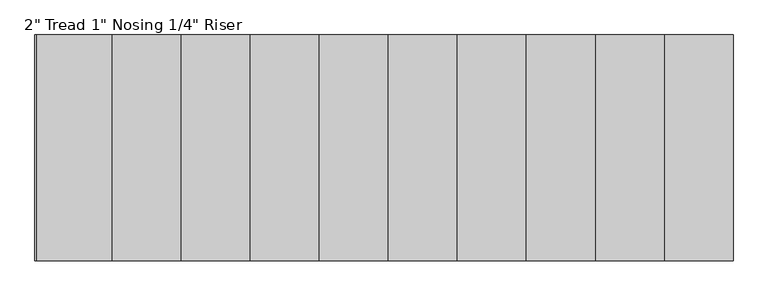
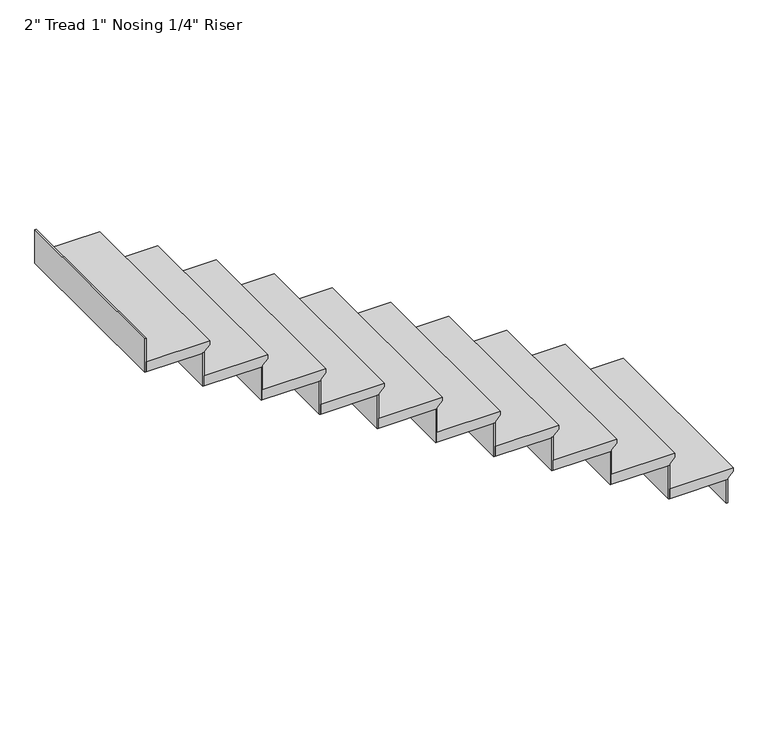
"""IFC4 building model written with IfcOpenShell, lengths in millimetres: stair flight geometry."""

from ifc_helpers import new_model, si_unit, origin, place, context, project, spatial, faceted_brep, source, transform, mapped, element, save


def stair_flight_26c172ca(model_context):
    return source(origin(), model_context, "Body", "Brep", [
        faceted_brep([(-5990.8517085, 2919.0826226, 455.0833333), (-5990.8517085, 2919.0826226, 474.1333333), (-5990.8517085, 2004.6826226, 474.1333333), (-5990.8517085, 2004.6826226, 455.0833333), (-6016.2517085, 2919.0826226, 429.6833333), (-6016.2517085, 2004.6826226, 429.6833333), (-6295.6517085, 2919.0826226, 474.1333333), (-6295.6517085, 2004.6826226, 474.1333333), (-6016.2517085, 2004.6826226, 423.3333333), (-6295.6517085, 2004.6826226, 423.3333333), (-6295.6517085, 2919.0826226, 423.3333333), (-6016.2517085, 2919.0826226, 423.3333333)], [[[0, 1, 2, 3]], [[4, 0, 3, 5]], [[2, 1, 6, 7]], [[8, 9, 10, 11]], [[2, 7, 9, 8, 5, 3]], [[8, 11, 4, 5]], [[6, 1, 0, 4, 11, 10]], [[7, 6, 10, 9]]]),
        faceted_brep([(-6016.2517085, 2919.0826226, 423.3333333), (-6016.2517085, 2919.0826226, 304.8), (-6022.6017085, 2919.0826226, 304.8), (-6022.6017085, 2919.0826226, 423.3333333), (-6016.2517085, 2004.6826226, 423.3333333), (-6022.6017085, 2004.6826226, 423.3333333), (-6022.6017085, 2004.6826226, 304.8), (-6016.2517085, 2004.6826226, 304.8)], [[[0, 1, 2, 3]], [[4, 5, 6, 7]], [[1, 0, 4, 7]], [[2, 1, 7, 6]], [[3, 2, 6, 5]], [[0, 3, 5, 4]]]),
        faceted_brep([(-6295.6517085, 2919.0826226, 592.6666667), (-6295.6517085, 2919.0826226, 423.3333333), (-6302.0017085, 2919.0826226, 423.3333333), (-6302.0017085, 2919.0826226, 592.6666667), (-6295.6517085, 2004.6826226, 592.6666667), (-6302.0017085, 2004.6826226, 592.6666667), (-6302.0017085, 2004.6826226, 423.3333333), (-6295.6517085, 2004.6826226, 423.3333333)], [[[0, 1, 2, 3]], [[4, 5, 6, 7]], [[1, 0, 4, 7]], [[2, 1, 7, 6]], [[3, 2, 6, 5]], [[0, 3, 5, 4]]]),
        faceted_brep([(-6270.2517085, 2004.6826226, 643.4666667), (-6270.2517085, 2919.0826226, 643.4666667), (-6575.0517085, 2919.0826226, 643.4666667), (-6575.0517085, 2004.6826226, 643.4666667), (-6295.6517085, 2004.6826226, 592.6666667), (-6575.0517085, 2004.6826226, 592.6666667), (-6575.0517085, 2919.0826226, 592.6666667), (-6295.6517085, 2919.0826226, 592.6666667), (-6295.6517085, 2004.6826226, 599.0166667), (-6270.2517085, 2004.6826226, 624.4166667), (-6295.6517085, 2919.0826226, 599.0166667), (-6270.2517085, 2919.0826226, 624.4166667)], [[[0, 1, 2, 3]], [[4, 5, 6, 7]], [[0, 3, 5, 4, 8, 9]], [[4, 7, 10, 8]], [[2, 1, 11, 10, 7, 6]], [[3, 2, 6, 5]], [[11, 1, 0, 9]], [[10, 11, 9, 8]]]),
        faceted_brep([(-6575.0517085, 2919.0826226, 762.0), (-6575.0517085, 2919.0826226, 592.6666667), (-6581.4017085, 2919.0826226, 592.6666667), (-6581.4017085, 2919.0826226, 762.0), (-6575.0517085, 2004.6826226, 762.0), (-6581.4017085, 2004.6826226, 762.0), (-6581.4017085, 2004.6826226, 592.6666667), (-6575.0517085, 2004.6826226, 592.6666667)], [[[0, 1, 2, 3]], [[4, 5, 6, 7]], [[1, 0, 4, 7]], [[2, 1, 7, 6]], [[3, 2, 6, 5]], [[0, 3, 5, 4]]]),
        faceted_brep([(-6549.6517085, 2004.6826226, 812.8), (-6549.6517085, 2919.0826226, 812.8), (-6854.4517085, 2919.0826226, 812.8), (-6854.4517085, 2004.6826226, 812.8), (-6575.0517085, 2004.6826226, 762.0), (-6854.4517085, 2004.6826226, 762.0), (-6854.4517085, 2919.0826226, 762.0), (-6575.0517085, 2919.0826226, 762.0), (-6575.0517085, 2004.6826226, 768.35), (-6549.6517085, 2004.6826226, 793.75), (-6575.0517085, 2919.0826226, 768.35), (-6549.6517085, 2919.0826226, 793.75)], [[[0, 1, 2, 3]], [[4, 5, 6, 7]], [[0, 3, 5, 4, 8, 9]], [[4, 7, 10, 8]], [[2, 1, 11, 10, 7, 6]], [[3, 2, 6, 5]], [[11, 1, 0, 9]], [[10, 11, 9, 8]]]),
        faceted_brep([(-6854.4517085, 2919.0826226, 931.3333333), (-6854.4517085, 2919.0826226, 762.0), (-6860.8017085, 2919.0826226, 762.0), (-6860.8017085, 2919.0826226, 931.3333333), (-6854.4517085, 2004.6826226, 931.3333333), (-6860.8017085, 2004.6826226, 931.3333333), (-6860.8017085, 2004.6826226, 762.0), (-6854.4517085, 2004.6826226, 762.0)], [[[0, 1, 2, 3]], [[4, 5, 6, 7]], [[1, 0, 4, 7]], [[2, 1, 7, 6]], [[3, 2, 6, 5]], [[0, 3, 5, 4]]]),
        faceted_brep([(-6829.0517085, 2004.6826226, 982.1333333), (-6829.0517085, 2919.0826226, 982.1333333), (-7133.8517085, 2919.0826226, 982.1333333), (-7133.8517085, 2004.6826226, 982.1333333), (-6854.4517085, 2004.6826226, 931.3333333), (-7133.8517085, 2004.6826226, 931.3333333), (-7133.8517085, 2919.0826226, 931.3333333), (-6854.4517085, 2919.0826226, 931.3333333), (-6854.4517085, 2004.6826226, 937.6833333), (-6829.0517085, 2004.6826226, 963.0833333), (-6854.4517085, 2919.0826226, 937.6833333), (-6829.0517085, 2919.0826226, 963.0833333)], [[[0, 1, 2, 3]], [[4, 5, 6, 7]], [[0, 3, 5, 4, 8, 9]], [[4, 7, 10, 8]], [[2, 1, 11, 10, 7, 6]], [[3, 2, 6, 5]], [[11, 1, 0, 9]], [[10, 11, 9, 8]]]),
        faceted_brep([(-7133.8517085, 2919.0826226, 1100.6666667), (-7133.8517085, 2919.0826226, 931.3333333), (-7140.2017085, 2919.0826226, 931.3333333), (-7140.2017085, 2919.0826226, 1100.6666667), (-7133.8517085, 2004.6826226, 1100.6666667), (-7140.2017085, 2004.6826226, 1100.6666667), (-7140.2017085, 2004.6826226, 931.3333333), (-7133.8517085, 2004.6826226, 931.3333333)], [[[0, 1, 2, 3]], [[4, 5, 6, 7]], [[1, 0, 4, 7]], [[2, 1, 7, 6]], [[3, 2, 6, 5]], [[0, 3, 5, 4]]]),
        faceted_brep([(-7108.4517085, 2004.6826226, 1151.4666667), (-7108.4517085, 2919.0826226, 1151.4666667), (-7413.2517085, 2919.0826226, 1151.4666667), (-7413.2517085, 2004.6826226, 1151.4666667), (-7133.8517085, 2004.6826226, 1100.6666667), (-7413.2517085, 2004.6826226, 1100.6666667), (-7413.2517085, 2919.0826226, 1100.6666667), (-7133.8517085, 2919.0826226, 1100.6666667), (-7133.8517085, 2004.6826226, 1107.0166667), (-7108.4517085, 2004.6826226, 1132.4166667), (-7133.8517085, 2919.0826226, 1107.0166667), (-7108.4517085, 2919.0826226, 1132.4166667)], [[[0, 1, 2, 3]], [[4, 5, 6, 7]], [[0, 3, 5, 4, 8, 9]], [[4, 7, 10, 8]], [[2, 1, 11, 10, 7, 6]], [[3, 2, 6, 5]], [[11, 1, 0, 9]], [[10, 11, 9, 8]]]),
        faceted_brep([(-7413.2517085, 2919.0826226, 1270.0), (-7413.2517085, 2919.0826226, 1100.6666667), (-7419.6017085, 2919.0826226, 1100.6666667), (-7419.6017085, 2919.0826226, 1270.0), (-7413.2517085, 2004.6826226, 1270.0), (-7419.6017085, 2004.6826226, 1270.0), (-7419.6017085, 2004.6826226, 1100.6666667), (-7413.2517085, 2004.6826226, 1100.6666667)], [[[0, 1, 2, 3]], [[4, 5, 6, 7]], [[1, 0, 4, 7]], [[2, 1, 7, 6]], [[3, 2, 6, 5]], [[0, 3, 5, 4]]]),
        faceted_brep([(-7387.8517085, 2004.6826226, 1320.8), (-7387.8517085, 2919.0826226, 1320.8), (-7692.6517085, 2919.0826226, 1320.8), (-7692.6517085, 2004.6826226, 1320.8), (-7413.2517085, 2004.6826226, 1270.0), (-7692.6517085, 2004.6826226, 1270.0), (-7692.6517085, 2919.0826226, 1270.0), (-7413.2517085, 2919.0826226, 1270.0), (-7413.2517085, 2004.6826226, 1276.35), (-7387.8517085, 2004.6826226, 1301.75), (-7413.2517085, 2919.0826226, 1276.35), (-7387.8517085, 2919.0826226, 1301.75)], [[[0, 1, 2, 3]], [[4, 5, 6, 7]], [[0, 3, 5, 4, 8, 9]], [[4, 7, 10, 8]], [[2, 1, 11, 10, 7, 6]], [[3, 2, 6, 5]], [[11, 1, 0, 9]], [[10, 11, 9, 8]]]),
        faceted_brep([(-7692.6517085, 2919.0826226, 1439.3333333), (-7692.6517085, 2919.0826226, 1270.0), (-7699.0017085, 2919.0826226, 1270.0), (-7699.0017085, 2919.0826226, 1439.3333333), (-7692.6517085, 2004.6826226, 1439.3333333), (-7699.0017085, 2004.6826226, 1439.3333333), (-7699.0017085, 2004.6826226, 1270.0), (-7692.6517085, 2004.6826226, 1270.0)], [[[0, 1, 2, 3]], [[4, 5, 6, 7]], [[1, 0, 4, 7]], [[2, 1, 7, 6]], [[3, 2, 6, 5]], [[0, 3, 5, 4]]]),
        faceted_brep([(-7667.2517085, 2004.6826226, 1490.1333333), (-7667.2517085, 2919.0826226, 1490.1333333), (-7972.0517085, 2919.0826226, 1490.1333333), (-7972.0517085, 2004.6826226, 1490.1333333), (-7692.6517085, 2004.6826226, 1439.3333333), (-7972.0517085, 2004.6826226, 1439.3333333), (-7972.0517085, 2919.0826226, 1439.3333333), (-7692.6517085, 2919.0826226, 1439.3333333), (-7692.6517085, 2004.6826226, 1445.6833333), (-7667.2517085, 2004.6826226, 1471.0833333), (-7692.6517085, 2919.0826226, 1445.6833333), (-7667.2517085, 2919.0826226, 1471.0833333)], [[[0, 1, 2, 3]], [[4, 5, 6, 7]], [[0, 3, 5, 4, 8, 9]], [[4, 7, 10, 8]], [[2, 1, 11, 10, 7, 6]], [[3, 2, 6, 5]], [[11, 1, 0, 9]], [[10, 11, 9, 8]]]),
        faceted_brep([(-7972.0517085, 2919.0826226, 1608.6666667), (-7972.0517085, 2919.0826226, 1439.3333333), (-7978.4017085, 2919.0826226, 1439.3333333), (-7978.4017085, 2919.0826226, 1608.6666667), (-7972.0517085, 2004.6826226, 1608.6666667), (-7978.4017085, 2004.6826226, 1608.6666667), (-7978.4017085, 2004.6826226, 1439.3333333), (-7972.0517085, 2004.6826226, 1439.3333333)], [[[0, 1, 2, 3]], [[4, 5, 6, 7]], [[1, 0, 4, 7]], [[2, 1, 7, 6]], [[3, 2, 6, 5]], [[0, 3, 5, 4]]]),
        faceted_brep([(-7946.6517085, 2004.6826226, 1659.4666667), (-7946.6517085, 2919.0826226, 1659.4666667), (-8251.4517085, 2919.0826226, 1659.4666667), (-8251.4517085, 2004.6826226, 1659.4666667), (-7972.0517085, 2004.6826226, 1608.6666667), (-8251.4517085, 2004.6826226, 1608.6666667), (-8251.4517085, 2919.0826226, 1608.6666667), (-7972.0517085, 2919.0826226, 1608.6666667), (-7972.0517085, 2004.6826226, 1615.0166667), (-7946.6517085, 2004.6826226, 1640.4166667), (-7972.0517085, 2919.0826226, 1615.0166667), (-7946.6517085, 2919.0826226, 1640.4166667)], [[[0, 1, 2, 3]], [[4, 5, 6, 7]], [[0, 3, 5, 4, 8, 9]], [[4, 7, 10, 8]], [[2, 1, 11, 10, 7, 6]], [[3, 2, 6, 5]], [[11, 1, 0, 9]], [[10, 11, 9, 8]]]),
        faceted_brep([(-8251.4517085, 2919.0826226, 1778.0), (-8251.4517085, 2919.0826226, 1608.6666667), (-8257.8017085, 2919.0826226, 1608.6666667), (-8257.8017085, 2919.0826226, 1778.0), (-8251.4517085, 2004.6826226, 1778.0), (-8257.8017085, 2004.6826226, 1778.0), (-8257.8017085, 2004.6826226, 1608.6666667), (-8251.4517085, 2004.6826226, 1608.6666667)], [[[0, 1, 2, 3]], [[4, 5, 6, 7]], [[1, 0, 4, 7]], [[2, 1, 7, 6]], [[3, 2, 6, 5]], [[0, 3, 5, 4]]]),
        faceted_brep([(-8226.0517085, 2004.6826226, 1828.8), (-8226.0517085, 2919.0826226, 1828.8), (-8530.8517085, 2919.0826226, 1828.8), (-8530.8517085, 2004.6826226, 1828.8), (-8251.4517085, 2004.6826226, 1778.0), (-8530.8517085, 2004.6826226, 1778.0), (-8530.8517085, 2919.0826226, 1778.0), (-8251.4517085, 2919.0826226, 1778.0), (-8251.4517085, 2004.6826226, 1784.35), (-8226.0517085, 2004.6826226, 1809.75), (-8251.4517085, 2919.0826226, 1784.35), (-8226.0517085, 2919.0826226, 1809.75)], [[[0, 1, 2, 3]], [[4, 5, 6, 7]], [[0, 3, 5, 4, 8, 9]], [[4, 7, 10, 8]], [[2, 1, 11, 10, 7, 6]], [[3, 2, 6, 5]], [[11, 1, 0, 9]], [[10, 11, 9, 8]]]),
        faceted_brep([(-8810.2517085, 2919.0826226, 2116.6666667), (-8810.2517085, 2919.0826226, 1947.3333333), (-8816.6017085, 2919.0826226, 1947.3333333), (-8816.6017085, 2919.0826226, 2116.6666667), (-8810.2517085, 2004.6826226, 2116.6666667), (-8816.6017085, 2004.6826226, 2116.6666667), (-8816.6017085, 2004.6826226, 1947.3333333), (-8810.2517085, 2004.6826226, 1947.3333333)], [[[0, 1, 2, 3]], [[4, 5, 6, 7]], [[1, 0, 4, 7]], [[2, 1, 7, 6]], [[3, 2, 6, 5]], [[0, 3, 5, 4]]]),
        faceted_brep([(-8530.8517085, 2919.0826226, 1947.3333333), (-8530.8517085, 2919.0826226, 1778.0), (-8537.2017085, 2919.0826226, 1778.0), (-8537.2017085, 2919.0826226, 1947.3333333), (-8530.8517085, 2004.6826226, 1947.3333333), (-8537.2017085, 2004.6826226, 1947.3333333), (-8537.2017085, 2004.6826226, 1778.0), (-8530.8517085, 2004.6826226, 1778.0)], [[[0, 1, 2, 3]], [[4, 5, 6, 7]], [[1, 0, 4, 7]], [[2, 1, 7, 6]], [[3, 2, 6, 5]], [[0, 3, 5, 4]]]),
        faceted_brep([(-8505.4517085, 2004.6826226, 1998.1333333), (-8505.4517085, 2919.0826226, 1998.1333333), (-8784.8517085, 2919.0826226, 1998.1333333), (-8810.2517085, 2919.0826226, 1998.1333333), (-8810.2517085, 2004.6826226, 1998.1333333), (-8530.8517085, 2004.6826226, 1947.3333333), (-8810.2517085, 2004.6826226, 1947.3333333), (-8810.2517085, 2919.0826226, 1947.3333333), (-8784.8517085, 2919.0826226, 1947.3333333), (-8530.8517085, 2919.0826226, 1947.3333333), (-8530.8517085, 2004.6826226, 1953.6833333), (-8505.4517085, 2004.6826226, 1979.0833333), (-8530.8517085, 2919.0826226, 1953.6833333), (-8505.4517085, 2919.0826226, 1979.0833333)], [[[0, 1, 2, 3, 4]], [[5, 6, 7, 8, 9]], [[0, 4, 6, 5, 10, 11]], [[5, 9, 12, 10]], [[2, 1, 13, 12, 9, 8]], [[3, 2, 8, 7]], [[4, 3, 7, 6]], [[13, 1, 0, 11]], [[12, 13, 11, 10]]]),
    ])


if __name__ == "__main__":
    model = new_model("IFC4")
    model_context = context("Model", 3, world=origin())
    ifc_project = project(units=[si_unit("LENGTHUNIT", "METRE", prefix="MILLI")], contexts=[model_context])
    site = spatial("IfcSite", under=ifc_project)
    building = spatial("IfcBuilding", under=site)
    placement = place(None, origin())
    stair_flight_shape = stair_flight_26c172ca(model_context)
    element("IfcStairFlight", 1, ObjectType="2\" Tread 1\" Nosing 1/4\" Riser", at=placement, inside=building, context=model_context, shape_type="MappedRepresentation", body=[
        mapped(stair_flight_shape, transform((0.0, 0.0, 0.0), x_axis=(1.0, 0.0, 0.0), y_axis=(0.0, 1.0, 0.0), z_axis=(0.0, 0.0, 1.0))),
    ])
    save(model, "model.ifc")
